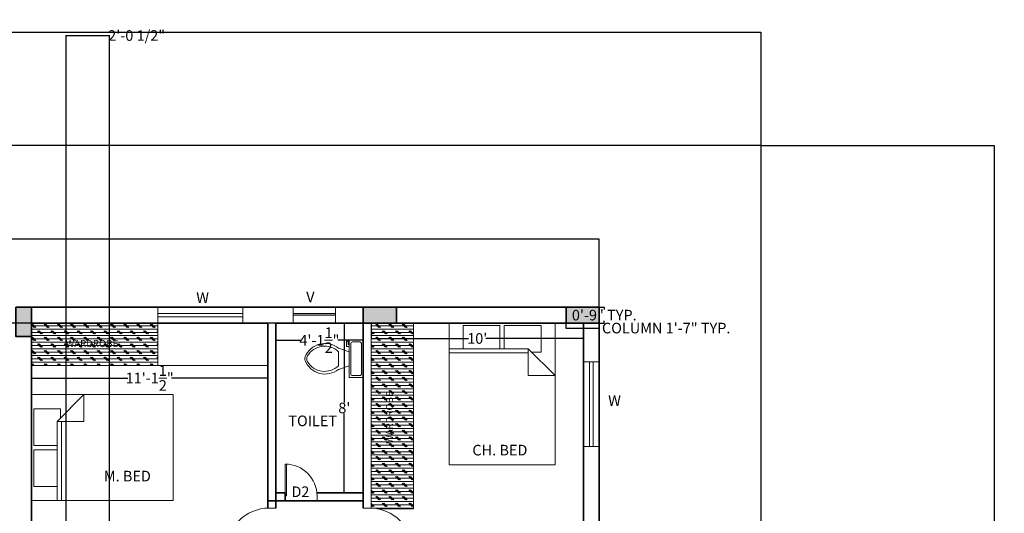
# Model space of a CAD drawing. Units: inches. Extents: x -2181 to 1225, y -80 to 4016.
# Tile 10 of 10: x 668 to 1225, y 456 to 736. Entities that reach past the tile are written whole.
import ezdxf

# ---------------------------------------------------------------- set-up
doc = ezdxf.new("R2010")
doc.units = ezdxf.units.IN
doc.header["$MEASUREMENT"] = 0
for name, color, linetype, lineweight in [('A-ANNO-DIMS', 2, 'Continuous', 18), ('A-ANNO-TEXT', 7, 'Continuous', 18), ('A-AREA-IDEN', 7, 'Continuous', 18), ('A-COLS', 7, 'Continuous', 35), ('A-COLS-PATT', 252, 'Continuous', 13), ('A-DOOR', 3, 'Continuous', 18), ('A-FLOR-FIXT', 8, 'Continuous', 18), ('A-FURN', 30, 'Continuous', 18), ('A-GLAZ', 4, 'Continuous', 18), ('A-GLAZ-PATT', 4, 'Continuous', 13), ('A-MILL', 8, 'Continuous', 18), ('A-MILL-PATT', 252, 'Continuous', 13), ('A-WALL', 7, 'Continuous', 35), ('C-PROP', 7, 'Continuous', 30)]:
    doc.layers.add(name, color=color, linetype=linetype, lineweight=lineweight)
doc.styles.get("Standard").update_dxf_attribs({"font": 'arial.ttf'})
doc.dimstyles.get("Standard").update_dxf_attribs({"dimtxt": 6, "dimasz": 0.18, "dimexe": 0.18, "dimexo": 0.0625, "dimgap": 0.09, "dimtad": 0, "dimtih": 1, "dimtoh": 1, "dimdec": 4, "dimzin": 0, "dimdsep": 46, "dimlunit": 4, "dimtxsty": 'Standard', "dimcen": 0.09, "dimadec": 0, "dimazin": 0, "dimtfac": 1, "dimtdec": 4, "dimtofl": 0, "dimtmove": 0, "dimatfit": 3, "dimfxl": 1, "dimtolj": 1, "dimtzin": 0, "dimarcsym": 0})
pattern_1 = [(0, (0, 0), (0, 1.875), []), (135, (0.9375, -0.9375), (-3.75, -3.75), [2.65165, -2.65165]), (135, (1.406, -0.9375), (-3.75, -3.75), [2.65165, -2.65165]), (135, (1.875, -0.9375), (-3.75, -3.75), [2.65165, -2.65165])]

# ---------------------------------------------------------------- blocks, each defined once
blk = doc.blocks.new('*U2')
for p, q in [((0, 0), (0, -6)), ((40, 0), (40, -6))]:
    blk.add_line(p, q)
blk.add_lwpolyline([(0, 0), (0, 40), (1.75, 40), (1.75, 0)], close=True)
blk.add_arc((0, 0), 40, 0, 90)
blk = doc.blocks.new('*U21')
for p, q in [((9.5, -6), (9.5, -2)), ((-10, -8.5), (-8, -8.5)), ((-10, -9.5), (-10, -8.5)), ((-7, -9.5), (-10, -9.5)), ((-8, -8.5), (-8, -8)), ((-7, -8), (-7, -9.5)), ((-4, -8), (-6, -14)), ((4, -8), (6, -14)), ((4, -14), (-4, -14))]:
    blk.add_line(p, q)
blk.add_lwpolyline([(10.5, -8), (10.5, 0), (-10.5, 0), (-10.5, -8)], close=True)
for points in [[(-9.5, -2), (-9.5, -6)], [(8.5, -1), (-8.5, -1)], [(-8.5, -7), (8.5, -7)]]:
    blk.add_lwpolyline(points)
for centre, radius, start, end in [((-8.62, -1.88), 0.884, 81.8699, 188.1301), ((8.62, -1.88), 0.884, 351.8699, 98.1301), ((-8.62, -6.12), 0.884, 171.8699, 278.1301), ((8.62, -6.12), 0.884, 261.8699, 8.1301), ((3.52, -21.58), 12.17, 141.4691, 247.9714), ((4.2, -21.82), 11.33, 136.3677, 238.9468), ((-3.52, -21.58), 12.17, 292.0284, 38.5307), ((-4.2, -21.82), 11.33, 301.053, 43.6321), ((0, -27.88), 4, 245.7318, 294.2682), ((0, -29), 4, 254.8605, 285.1395)]:
    blk.add_arc(centre, radius, start, end)
blk = doc.blocks.new('Bed - Queen')
for p, q in [((0, -80.00003), (0, 0)), ((0, 0), (59.99999, 0)), ((59.99999, 0), (59.99999, -80.00003)), ((7.99999, -1.2), (28.79998, -1.2)), ((7.99999, -14.4), (7.99999, -1.2)), ((28.79998, -1.2), (28.79998, -14.4)), ((31.19999, -1.2), (51.99999, -1.2)), ((31.19999, -14.4), (31.19999, -1.2)), ((51.99999, -1.2), (51.99999, -16.4)), ((0, -14.4), (44.8, -14.4)), ((59.99999, -29.6), (44.8, -14.4)), ((44.8, -14.4), (44.8, -29.6)), ((51.99999, -16.4), (46.79936, -16.4)), ((44.8, -16.8), (0, -16.8)), ((44.8, -29.6), (59.99999, -29.6)), ((59.99999, -80.00003), (0, -80.00003))]:
    blk.add_line(p, q)
blk = doc.blocks.new('*D50')
at = {"layer": 'A-ANNO-DIMS', "color": 0, "lineweight": -2, "transparency": 16777216}
for p, q in [((674.51, 563.92), (674.51, 532.72)), ((808.01, 563.92), (808.01, 532.72)), ((674.69, 532.9), (728.96, 532.9)), ((807.83, 532.9), (753.57, 532.9))]:
    blk.add_line(p, q, dxfattribs=at)
at = {"layer": 'A-ANNO-DIMS', "color": 0, "transparency": 16777216}
for points in [[(674.69, 532.93), (674.69, 532.87), (674.51, 532.9)], [(807.83, 532.93), (807.83, 532.87), (808.01, 532.9)]]:
    blk.add_solid(points, dxfattribs=at)
at = {"layer": 'Defpoints', "color": 0, "transparency": 16777216}
for p in [(674.51, 563.98), (808.01, 563.98), (808.01, 532.9)]:
    blk.add_point(p, dxfattribs=at)
at = {"layer": 'A-ANNO-DIMS', "color": 0, "transparency": 16777216, "insert": (741.26, 532.9), "char_height": 6, "attachment_point": 5}
blk.add_mtext('\\A1;11\'-1{\\H1x;\\S1/2;}"', dxfattribs=at)
blk = doc.blocks.new('*D63')
at = {"layer": 'A-ANNO-DIMS', "color": 0, "lineweight": -2, "transparency": 16777216}
for p, q in [((866.51, 563.92), (866.51, 555.11)), ((986.51, 563.92), (986.51, 555.11)), ((866.69, 555.29), (921.62, 555.29)), ((986.33, 555.29), (931.41, 555.29))]:
    blk.add_line(p, q, dxfattribs=at)
at = {"layer": 'A-ANNO-DIMS', "color": 0, "transparency": 16777216}
for points in [[(866.69, 555.32), (866.69, 555.26), (866.51, 555.29)], [(986.33, 555.32), (986.33, 555.26), (986.51, 555.29)]]:
    blk.add_solid(points, dxfattribs=at)
at = {"layer": 'Defpoints', "color": 0, "transparency": 16777216}
for p in [(866.51, 563.98), (986.51, 563.98), (986.51, 555.29)]:
    blk.add_point(p, dxfattribs=at)
at = {"layer": 'A-ANNO-DIMS', "color": 0, "transparency": 16777216, "insert": (926.51, 555.29), "char_height": 6, "attachment_point": 5}
blk.add_mtext("\\A1;10'", dxfattribs=at)
blk = doc.blocks.new('*D64')
at = {"layer": 'A-ANNO-DIMS', "color": 0, "lineweight": -2, "transparency": 16777216}
for p, q in [((812.51, 563.92), (812.51, 554.11)), ((862.01, 563.92), (862.01, 554.11)), ((812.69, 554.29), (826.89, 554.29)), ((861.83, 554.29), (847.64, 554.29))]:
    blk.add_line(p, q, dxfattribs=at)
at = {"layer": 'A-ANNO-DIMS', "color": 0, "transparency": 16777216}
for points in [[(812.69, 554.32), (812.69, 554.26), (812.51, 554.29)], [(861.83, 554.32), (861.83, 554.26), (862.01, 554.29)]]:
    blk.add_solid(points, dxfattribs=at)
at = {"layer": 'Defpoints', "color": 0, "transparency": 16777216}
for p in [(812.51, 563.98), (862.01, 563.98), (862.01, 554.29)]:
    blk.add_point(p, dxfattribs=at)
at = {"layer": 'A-ANNO-DIMS', "color": 0, "transparency": 16777216, "insert": (837.26, 554.29), "char_height": 6, "attachment_point": 5}
blk.add_mtext('\\A1;4\'-1{\\H1x;\\S1/2;}"', dxfattribs=at)
blk = doc.blocks.new('*D65')
at = {"layer": 'A-ANNO-DIMS', "color": 0, "lineweight": -2, "transparency": 16777216}
for p, q in [((861.95, 563.98), (851.15, 563.98)), ((851.33, 563.8), (851.33, 519.14)), ((851.33, 468.16), (851.33, 512.83)), ((861.95, 467.98), (851.15, 467.98))]:
    blk.add_line(p, q, dxfattribs=at)
at = {"layer": 'A-ANNO-DIMS', "color": 0, "transparency": 16777216}
for points in [[(851.3, 563.8), (851.36, 563.8), (851.33, 563.98)], [(851.3, 468.16), (851.36, 468.16), (851.33, 467.98)]]:
    blk.add_solid(points, dxfattribs=at)
at = {"layer": 'Defpoints', "color": 0, "transparency": 16777216}
for p in [(851.33, 563.98), (862.01, 563.98), (862.01, 467.98)]:
    blk.add_point(p, dxfattribs=at)
at = {"layer": 'A-ANNO-DIMS', "color": 0, "transparency": 16777216, "insert": (851.33, 515.98), "char_height": 6, "attachment_point": 5}
blk.add_mtext("\\A1;8'", dxfattribs=at)
blk = doc.blocks.new('*D70')
at = {"layer": 'A-ANNO-DIMS', "color": 0, "lineweight": -2, "transparency": 16777216}
for p, q in [((7.01, 664.55), (7.01, 728.44)), ((7.19, 728.26), (541.83, 728.26)), ((1086.83, 728.26), (552.2, 728.26)), ((1087.01, 664.55), (1087.01, 728.44))]:
    blk.add_line(p, q, dxfattribs=at)
at = {"layer": 'A-ANNO-DIMS', "color": 0, "transparency": 16777216}
for points in [[(7.19, 728.29), (7.19, 728.23), (7.01, 728.26)], [(1086.83, 728.29), (1086.83, 728.23), (1087.01, 728.26)]]:
    blk.add_solid(points, dxfattribs=at)
at = {"layer": 'Defpoints', "color": 0, "transparency": 16777216}
for p in [(1087.01, 728.26), (7.01, 664.48), (1087.01, 664.48)]:
    blk.add_point(p, dxfattribs=at)
at = {"layer": 'A-ANNO-DIMS', "color": 0, "transparency": 16777216, "insert": (547.01, 728.26), "char_height": 6, "attachment_point": 5}
blk.add_mtext("\\A1;90'", dxfattribs=at)
blk = doc.blocks.new('*D71')
at = {"layer": 'A-ANNO-DIMS', "color": 0, "lineweight": -2, "transparency": 16777216}
for p, q in [((98.51, 573.05), (98.51, 611.58)), ((98.69, 611.4), (536.64, 611.4)), ((995.33, 611.4), (557.39, 611.4)), ((995.51, 573.05), (995.51, 611.58))]:
    blk.add_line(p, q, dxfattribs=at)
at = {"layer": 'A-ANNO-DIMS', "color": 0, "transparency": 16777216}
for points in [[(98.69, 611.43), (98.69, 611.37), (98.51, 611.4)], [(995.33, 611.43), (995.33, 611.37), (995.51, 611.4)]]:
    blk.add_solid(points, dxfattribs=at)
at = {"layer": 'Defpoints', "color": 0, "transparency": 16777216}
for p in [(995.51, 611.4), (98.51, 572.98), (995.51, 572.98)]:
    blk.add_point(p, dxfattribs=at)
at = {"layer": 'A-ANNO-DIMS', "color": 0, "transparency": 16777216, "insert": (547.01, 611.4), "char_height": 6, "attachment_point": 5}
blk.add_mtext('\\A1;74\'-9"', dxfattribs=at)
blk = doc.blocks.new('*D73')
at = {"layer": 'A-ANNO-DIMS', "color": 0, "lineweight": -2, "transparency": 16777216}
for p, q in [((1087.08, 664.48), (1219.08, 664.48)), ((1218.9, 664.3), (1218.9, 343.63)), ((1218.9, 16.66), (1218.9, 337.34)), ((1087.08, 16.48), (1219.08, 16.48))]:
    blk.add_line(p, q, dxfattribs=at)
at = {"layer": 'A-ANNO-DIMS', "color": 0, "transparency": 16777216}
for points in [[(1218.87, 664.3), (1218.93, 664.3), (1218.9, 664.48)], [(1218.87, 16.66), (1218.93, 16.66), (1218.9, 16.48)]]:
    blk.add_solid(points, dxfattribs=at)
at = {"layer": 'Defpoints', "color": 0, "transparency": 16777216}
for p in [(1087.01, 664.48), (1218.9, 664.48), (1087.01, 16.48)]:
    blk.add_point(p, dxfattribs=at)
at = {"layer": 'A-ANNO-DIMS', "color": 0, "transparency": 16777216, "insert": (1218.9, 340.48), "char_height": 6, "attachment_point": 5}
blk.add_mtext("\\A1;54'", dxfattribs=at)
blk = doc.blocks.new('COL-16.5X9')
blk.add_lwpolyline([(0, 16.5), (9, 16.5), (9, 0), (0, 0)], close=True)
blk = doc.blocks.new('COL-18.81X9')
blk.add_lwpolyline([(0, 9), (18.81, 9), (18.81, 0), (0, 0)], close=True)
blk = doc.blocks.new('WIN-48')
for p, q in [((0, 9), (0, 0)), ((48, 9), (48, 0)), ((0, 5.5), (48, 5.5)), ((0, 3.5), (48, 3.5))]:
    blk.add_line(p, q)
blk = doc.blocks.new('*D116')
at = {"layer": 'A-ANNO-DIMS', "color": 0, "lineweight": -2, "transparency": 16777216}
for p, q in [((976.7, 563.92), (976.7, 560.98)), ((995.51, 563.92), (995.51, 560.98)), ((976.88, 561.16), (995.33, 561.16)), ((995.51, 561.16), (995.69, 561.16))]:
    blk.add_line(p, q, dxfattribs=at)
at = {"layer": 'A-ANNO-DIMS', "color": 0, "transparency": 16777216}
for points in [[(976.88, 561.19), (976.88, 561.13), (976.7, 561.16)], [(995.33, 561.19), (995.33, 561.13), (995.51, 561.16)]]:
    blk.add_solid(points, dxfattribs=at)
at = {"layer": 'Defpoints', "color": 0, "transparency": 16777216}
for p in [(976.7, 563.98), (995.51, 563.98), (995.51, 561.16)]:
    blk.add_point(p, dxfattribs=at)
at = {"layer": 'A-ANNO-DIMS', "color": 0, "transparency": 16777216, "insert": (1033.36, 561.16), "char_height": 6, "attachment_point": 5}
blk.add_mtext('\\A1;COLUMN 1\'-7" TYP.', dxfattribs=at)
blk = doc.blocks.new('*D117')
at = {"layer": 'A-ANNO-DIMS', "color": 0, "lineweight": -2, "transparency": 16777216}
for p, q in [((995.58, 572.98), (998.52, 572.98)), ((998.34, 572.8), (998.34, 571.64)), ((995.58, 563.98), (998.52, 563.98)), ((998.34, 564.16), (998.34, 565.33))]:
    blk.add_line(p, q, dxfattribs=at)
at = {"layer": 'A-ANNO-DIMS', "color": 0, "transparency": 16777216}
for points in [[(998.31, 572.8), (998.37, 572.8), (998.34, 572.98)], [(998.31, 564.16), (998.37, 564.16), (998.34, 563.98)]]:
    blk.add_solid(points, dxfattribs=at)
at = {"layer": 'Defpoints', "color": 0, "transparency": 16777216}
for p in [(995.51, 572.98), (998.34, 572.98), (995.51, 563.98)]:
    blk.add_point(p, dxfattribs=at)
at = {"layer": 'A-ANNO-DIMS', "color": 0, "transparency": 16777216, "insert": (998.34, 568.48), "char_height": 6, "attachment_point": 5}
blk.add_mtext('\\A1;0\'-9" TYP.', dxfattribs=at)
blk = doc.blocks.new('*D131')
at = {"layer": 'A-ANNO-DIMS', "color": 0, "lineweight": -2, "transparency": 16777216}
for p, q in [((976.64, 563.98), (-59.44, 563.98)), ((-59.26, 563.8), (-59.26, 500.43)), ((-59.26, 430.66), (-59.26, 494.04)), ((977.45, 430.48), (-59.44, 430.48))]:
    blk.add_line(p, q, dxfattribs=at)
at = {"layer": 'A-ANNO-DIMS', "color": 0, "transparency": 16777216}
for points in [[(-59.29, 563.8), (-59.23, 563.8), (-59.26, 563.98)], [(-59.29, 430.66), (-59.23, 430.66), (-59.26, 430.48)]]:
    blk.add_solid(points, dxfattribs=at)
at = {"layer": 'Defpoints', "color": 0, "transparency": 16777216}
for p in [(976.7, 563.98), (-59.26, 430.48), (977.51, 430.48)]:
    blk.add_point(p, dxfattribs=at)
at = {"layer": 'A-ANNO-DIMS', "color": 0, "transparency": 16777216, "insert": (-59.26, 497.23), "char_height": 6, "attachment_point": 5}
blk.add_mtext('\\A1;11\'-1 1/2"', dxfattribs=at)
blk = doc.blocks.new('*D134')
at = {"layer": 'A-ANNO-DIMS', "color": 0, "lineweight": -2, "transparency": 16777216}
for p, q in [((693.95, 426.05), (693.95, 726.81)), ((694.13, 726.63), (718.45, 726.63)), ((718.63, 426.05), (718.63, 726.81)), ((718.63, 726.63), (718.81, 726.63))]:
    blk.add_line(p, q, dxfattribs=at)
at = {"layer": 'A-ANNO-DIMS', "color": 0, "transparency": 16777216}
for points in [[(694.13, 726.66), (694.13, 726.6), (693.95, 726.63)], [(718.45, 726.66), (718.45, 726.6), (718.63, 726.63)]]:
    blk.add_solid(points, dxfattribs=at)
at = {"layer": 'Defpoints', "color": 0, "transparency": 16777216}
for p in [(718.63, 726.63), (693.95, 425.98), (718.63, 425.98)]:
    blk.add_point(p, dxfattribs=at)
at = {"layer": 'A-ANNO-DIMS', "color": 0, "transparency": 16777216, "insert": (733.91, 726.63), "char_height": 6, "attachment_point": 5}
blk.add_mtext('\\A1;2\'-0 1/2"', dxfattribs=at)

msp = doc.modelspace()

# ---------------------------------------------------------------- hatches: boundary and pattern name
at = {"layer": 'A-COLS-PATT'}
h = msp.add_hatch(color=256, dxfattribs=at)
h.dxf.hatch_style = 1
h.paths.add_polyline_path([(995.51461, 209.98479), (986.51461, 209.98479), (986.51461, 191.48479), (995.51461, 191.48479)])
h.paths.add_polyline_path([(862.50488, 191.48479), (862.50488, 200.48479), (841.01461, 200.48479), (841.01461, 191.48479)])
h.paths.add_polyline_path([(995.51461, 425.98479), (995.51461, 434.98479), (977.51461, 434.98479), (977.51461, 425.98479)])
h.paths.add_polyline_path([(880.01461, 425.98479), (880.01461, 432.54138), (862.01461, 432.54138), (862.01461, 425.98479)])
h.paths.add_polyline_path([(880.82546, 563.98479), (880.82546, 572.98479), (862.01461, 572.98479), (862.01461, 563.98479)])
h.paths.add_polyline_path([(995.51461, 563.98479), (995.51461, 572.98479), (976.70377, 572.98479), (976.70377, 563.98479)])
h.paths.add_polyline_path([(674.51461, 572.98479), (665.51461, 572.98479), (665.51461, 556.48479), (674.51461, 556.48479)])
h.paths.add_polyline_path([(674.51461, 442.48479), (665.51461, 442.48479), (665.51461, 425.98479), (674.51461, 425.98479)])
at = {"layer": 'A-GLAZ-PATT'}
h = msp.add_hatch(color=256, dxfattribs=at)
h.dxf.hatch_style = 1
h.paths.add_polyline_path([(846.43785, 569.48479), (822.43785, 569.48479), (822.43785, 568.48479), (846.43785, 568.48479)])
at = {"layer": 'A-MILL-PATT'}
h = msp.add_hatch(dxfattribs=at)
h.set_pattern_fill('CORK', color=256, scale=15)
h.set_pattern_definition(pattern_1)
h.paths.add_polyline_path([(674.51461, 563.98479), (674.51461, 539.98479), (745.86356, 539.98479), (745.86356, 563.98479)])
h = msp.add_hatch(dxfattribs=at)
h.set_pattern_fill('CORK', color=256, scale=15)
h.set_pattern_definition(pattern_1)
h.paths.add_polyline_path([(890.51461, 563.98479), (866.51461, 563.98479), (866.51461, 458.98479), (890.51461, 458.88288)])

# ---------------------------------------------------------------- linework, layer by layer
at = {"layer": 'A-COLS'}
msp.add_line((986.51461, 563.98479), (995.51461, 563.98479), dxfattribs=at)
msp.add_lwpolyline([(976.70377, 563.98479), (976.70377, 572.98479), (995.51461, 572.98479), (995.51461, 563.95842)], dxfattribs=at)
at = {"layer": 'A-GLAZ'}
for p, q in [((745.86356, 539.98479), (745.86356, 572.98479)), ((745.86356, 569.48479), (793.86356, 569.48479)), ((793.86356, 563.98479), (793.86356, 572.98479)), ((822.43785, 563.98479), (822.43785, 572.98479)), ((822.43785, 569.48479), (846.43785, 569.48479)), ((822.43785, 568.48479), (846.43785, 568.48479)), ((846.43785, 563.98479), (846.43785, 572.98479)), ((745.86356, 567.48479), (793.86356, 567.48479))]:
    msp.add_line(p, q, dxfattribs=at)
at = {"layer": 'A-MILL'}
for p, q in [((674.51461, 572.98479), (674.51461, 539.98479)), ((866.51461, 563.98479), (890.51461, 563.98479)), ((890.51461, 563.98479), (890.51461, 458.88288)), ((674.51461, 539.98479), (808.01461, 539.98479)), ((890.51461, 458.88288), (869.86898, 458.97054))]:
    msp.add_line(p, q, dxfattribs=at)
msp.add_lwpolyline([(866.51461, 459.32103), (866.51461, 563.98479)], dxfattribs=at)
at = {"layer": 'A-WALL'}
msp.add_line((817.88725, 467.98479), (817.88725, 463.48479), dxfattribs=at)
for points in [[(995.51461, 136.48479), (995.51461, 572.98479), (665.51461, 572.98479)], [(674.51461, 425.98479), (674.51461, 563.98479)], [(808.01461, 563.98479), (674.51461, 563.98479)], [(808.01461, 459.32103), (808.01461, 563.98479)], [(862.01461, 563.98479), (812.51461, 563.98479)], [(812.51461, 459.33578), (812.51461, 563.98479)], [(862.01461, 459.33578), (862.01461, 563.98479)], [(986.51461, 563.98479), (866.51461, 563.98479)], [(986.51461, 434.98479), (986.51461, 563.98479)], [(817.88725, 467.98479), (812.51461, 467.98479)], [(862.01461, 467.98479), (835.80955, 467.98479)], [(862.01461, 463.48479), (808.01461, 463.48479)]]:
    msp.add_lwpolyline(points, dxfattribs=at)
at = {"layer": 'C-PROP'}
msp.add_lwpolyline([(1087.01461, 16.48479), (1087.01461, 664.48479), (7.01461, 664.48479), (7.01461, 16.48479)], dxfattribs=at)

# ---------------------------------------------------------------- block references
at = {"layer": 'A-COLS'}
for name, p in [('COL-16.5X9', (665.515, 556.485)), ('COL-18.81X9', (976.704, 563.985))]:
    msp.add_blockref(name, p, dxfattribs=at)
at = {"layer": 'A-COLS', "extrusion": (0, 0, -1), "zscale": -1}
msp.add_blockref('COL-18.81X9', (-880.82523, 563.985), dxfattribs=at)
at = {"layer": 'A-DOOR', "xscale": 0.4503069535887608, "yscale": 0.4503069535887608, "zscale": 0.4503069535887608}
msp.add_blockref('*U2', (817.88725, 466.18663), dxfattribs=at)
at = {"layer": 'A-DOOR', "xscale": 0.608774911433326, "yscale": 0.608774911433326, "zscale": 0.608774911433326, "rotation": 90.00000000000003}
msp.add_blockref('*U2', (808.86196, 434.98479), dxfattribs=at)
at = {"layer": 'A-DOOR', "extrusion": (0, 0, -1), "xscale": 0.608774911433326, "yscale": 0.608774911433326, "zscale": -0.608774911433326, "rotation": 90.00000000000003}
msp.add_blockref('*U2', (-865.66726, 434.98479), dxfattribs=at)
at = {"layer": 'A-FLOR-FIXT', "rotation": 270}
msp.add_blockref('*U21', (862.01461, 543.79499), dxfattribs=at)
at = {"layer": 'A-FURN'}
msp.add_blockref('Bed - Queen', (910.56752, 563.87204), dxfattribs=at)
at = {"layer": 'A-FURN', "rotation": 90}
msp.add_blockref('Bed - Queen', (674.51461, 463.55197), dxfattribs=at)
at = {"layer": 'A-GLAZ', "extrusion": (0, 0, -1), "zscale": -1, "rotation": 269.9999999999998}
msp.add_blockref('WIN-48', (-995.5144, 542.13284), dxfattribs=at)

# ---------------------------------------------------------------- texts
at = {"layer": 'A-ANNO-TEXT', "attachment_point": 1}
for s, width, insert, char_height in [('W', 291.4178321, (767.6103, 581.35407), 6), ('V', 291.4178321, (829.77746, 581.76614), 6), ('WARDROBE', 13.1749235, (693.82971, 554.39038), 4), ('W', 291.4178321, (1000.54953, 523.13709), 6), ('D2', 291.4178321, (821.41139, 471.59063), 6)]:
    msp.add_mtext_dynamic_manual_height_columns(s, width=width, gutter_width=1, heights=[0], dxfattribs=dict(at, insert=insert, char_height=char_height))
at = {"layer": 'A-ANNO-TEXT', "insert": (874.89948, 495.73488), "char_height": 4, "attachment_point": 1, "rotation": 90}
msp.add_mtext_dynamic_manual_height_columns('WARDROBE', width=13.1749235, gutter_width=1, heights=[0], dxfattribs=at)
at = {"layer": 'A-AREA-IDEN', "char_height": 6, "attachment_point": 1}
for s, insert in [('TOILET', (819.65937, 511.68098)), ('CH. BED', (923.76124, 495.12903)), ('M. BED', (715.35329, 480.43442))]:
    msp.add_mtext_dynamic_manual_height_columns(s, width=291.4178321, gutter_width=1, heights=[0], dxfattribs=dict(at, insert=insert))

# ---------------------------------------------------------------- dimensions: what is measured, and where the dimension line sits
at = {"layer": 'A-ANNO-DIMS'}
for base, p1, p2, override, picture, middle in [((718.62706, 726.63478), (693.94574, 425.98478), (718.62706, 425.98478), {"dimdec": 1, "dimlfac": 1, "dimrnd": 0, "dimzin": 1, "dimdsep": 46, "dimlunit": 4, "dimfrac": 2}, '*D134', (733.91343, 726.63478)), ((1087.01461, 728.26231), (7.01461, 664.48479), (1087.01461, 664.48479), {"dimclrd": 0, "dimclre": 0, "dimclrt": 0}, '*D70', (547.01461, 728.26231)), ((995.51461, 611.40365), (98.51461, 572.98479), (995.51461, 572.98479), {"dimclrd": 0, "dimclre": 0, "dimclrt": 0}, '*D71', (547.01461, 611.40365)), ((808.01461, 532.89548), (674.51461, 563.98479), (808.01461, 563.98479), {"dimclrd": 0, "dimclre": 0, "dimclrt": 0}, '*D50', (741.26461, 532.89548)), ((862.01461, 554.29499), (812.51461, 563.98479), (862.01461, 563.98479), {"dimclrd": 0, "dimclre": 0, "dimclrt": 0}, '*D64', (837.26461, 554.29499)), ((986.51461, 555.29411), (866.51461, 563.98479), (986.51461, 563.98479), {"dimclrd": 0, "dimclre": 0, "dimclrt": 0}, '*D63', (926.51461, 555.29411))]:
    dim = msp.add_linear_dim(base=base, p1=p1, p2=p2, dimstyle='Standard', override=override, dxfattribs=at)
    dim.commit()
    dim.dimension.update_dxf_attribs({"geometry": picture, "text_midpoint": middle})
for base, p1, p2, override, picture, middle in [((1218.89961, 664.48479), (1087.01461, 16.48479), (1087.01461, 664.48479), {"dimclrd": 0, "dimclre": 0, "dimclrt": 0}, '*D73', (1218.89961, 340.48479)), ((-59.2566, 430.48478), (976.70377, 563.98478), (977.51461, 430.48478), {"dimdec": 1, "dimlfac": 1, "dimrnd": 0, "dimzin": 1, "dimdsep": 46, "dimlunit": 4, "dimfrac": 2}, '*D131', (-59.2566, 497.23478)), ((851.33455, 563.98479), (862.01461, 467.98479), (862.01461, 563.98479), {"dimclrd": 0, "dimclre": 0, "dimclrt": 0}, '*D65', (851.33455, 515.98479))]:
    dim = msp.add_linear_dim(base=base, p1=p1, p2=p2, angle=90, dimstyle='Standard', override=override, dxfattribs=at)
    dim.commit()
    dim.dimension.update_dxf_attribs({"geometry": picture, "text_midpoint": middle})
dim = msp.add_linear_dim(base=(995.51461, 561.16316), p1=(976.70377, 563.98479), p2=(995.51461, 563.98479), text='COLUMN <> TYP.', dimstyle='Standard', override={"dimdec": 1, "dimlfac": 1, "dimrnd": 0, "dimzin": 1, "dimdsep": 46, "dimlunit": 4, "dimfrac": 2}, dxfattribs=at)
dim.commit()
dim.dimension.update_dxf_attribs({"geometry": '*D116', "text_midpoint": (1033.36238, 561.16316)})
dim = msp.add_linear_dim(base=(998.33624, 572.98479), p1=(995.51461, 563.98479), p2=(995.51461, 572.98479), angle=90, text='<> TYP.', dimstyle='Standard', override={"dimdec": 1, "dimlfac": 1, "dimrnd": 0, "dimzin": 1, "dimdsep": 46, "dimlunit": 4, "dimfrac": 2}, dxfattribs=at)
dim.commit()
dim.dimension.update_dxf_attribs({"geometry": '*D117', "text_midpoint": (998.33624, 568.48479)})

doc.saveas('drawing.dxf')
